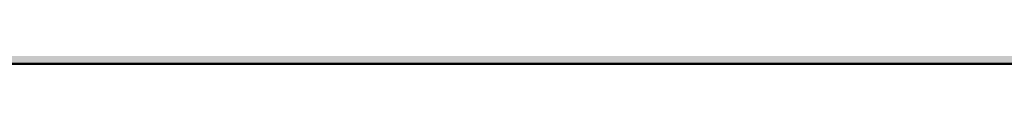
# Model space of a CAD drawing. Units: millimetres. Extents: x 0 to 2267, y 0 to 1823.
# Tile 213 of 256: x 1841.442 to 1842.748, y 1127.417 to 1127.417. Entities that reach past the tile are written whole.
import ezdxf

# ---------------------------------------------------------------- set-up
doc = ezdxf.new("R2010")
doc.units = ezdxf.units.MM
doc.header["$MEASUREMENT"] = 0
for name, color, linetype, lineweight in [('M-DIMS', 2, 'Continuous', 25), ('M-HATC', 252, 'Continuous', 18), ('M-OUTL', 7, 'Continuous', 50)]:
    doc.layers.add(name, color=color, linetype=linetype, lineweight=lineweight)
doc.styles.get("Standard").update_dxf_attribs({"font": 'arial.ttf'})
doc.dimstyles.get("Standard").update_dxf_attribs({"dimtxt": 7, "dimasz": 4, "dimexe": 0.18, "dimexo": 0.0625, "dimgap": 0.09, "dimtad": 0, "dimdec": 0, "dimzin": 0, "dimdsep": 46, "dimtxsty": 'Standard', "dimcen": 0.09, "dimadec": 0, "dimazin": 0, "dimtfac": 1, "dimtdec": 0, "dimtofl": 0, "dimtmove": 0, "dimatfit": 3, "dimfxl": 1, "dimtolj": 1, "dimtzin": 0, "dimarcsym": 0})

# ---------------------------------------------------------------- blocks, each defined once
blk = doc.blocks.new('*D1')
at = {"layer": 'Defpoints', "color": 0, "transparency": 16777216}
for p in [(1593.4289, 1127.4171), (1843.4289, 1127.4171), (1843.4289, 955.6278)]:
    blk.add_point(p, dxfattribs=at)
at = {"layer": 'M-DIMS', "color": 0, "lineweight": -2, "transparency": 16777216}
for p, q in [((1593.4289, 1127.3546), (1593.4289, 955.4478)), ((1843.4289, 1127.3546), (1843.4289, 955.4478)), ((1597.4289, 955.6278), (1710.5582, 955.6278)), ((1839.4289, 955.6278), (1726.2996, 955.6278))]:
    blk.add_line(p, q, dxfattribs=at)
at = {"layer": 'M-DIMS', "color": 0, "transparency": 16777216}
for points in [[(1597.4289, 956.2944), (1597.4289, 954.9611), (1593.4289, 955.6278)], [(1839.4289, 956.2944), (1839.4289, 954.9611), (1843.4289, 955.6278)]]:
    blk.add_solid(points, dxfattribs=at)
at = {"layer": 'M-DIMS', "color": 0, "transparency": 16777216, "insert": (1718.4289, 955.6278), "char_height": 7, "attachment_point": 5}
blk.add_mtext('\\A1;250', dxfattribs=at)

msp = doc.modelspace()

# ---------------------------------------------------------------- hatches: boundary and pattern name
at = {"layer": 'M-HATC'}
h = msp.add_hatch(color=256, dxfattribs=at)
h.dxf.hatch_style = 1
h.paths.add_polyline_path([(2042.8886, 1580.1796), (2055.771, 1593.062), (1381.0868, 1593.062), (1393.9692, 1580.1796), (1374.086, 1560.2964), (2062.7718, 1560.2964)])
h.paths.add_polyline_path([(1843.4289, 1201.3297), (1843.4289, 1227.2475), (1593.4289, 1227.2475), (1593.4289, 1201.3297, -0.228274), (1574.5989, 1162.2346), (1530.9289, 1127.4171), (1905.9289, 1127.4171), (1862.2589, 1162.2346, -0.228274)])

# ---------------------------------------------------------------- linework, layer by layer
at = {"layer": 'M-OUTL'}
msp.add_line((1530.9289, 1127.4171), (1905.9289, 1127.4171), dxfattribs=at)

# ---------------------------------------------------------------- dimensions: what is measured, and where the dimension line sits
at = {"layer": 'M-DIMS'}
dim = msp.add_linear_dim(base=(1843.4289, 955.6278), p1=(1593.4289, 1127.4171), p2=(1843.4289, 1127.4171), dimstyle='Standard', override={"dimclrd": 0, "dimclre": 0, "dimclrt": 0}, dxfattribs=at)
dim.commit()
dim.dimension.update_dxf_attribs({"geometry": '*D1', "text_midpoint": (1718.4289, 955.6278)})

doc.saveas('drawing.dxf')
